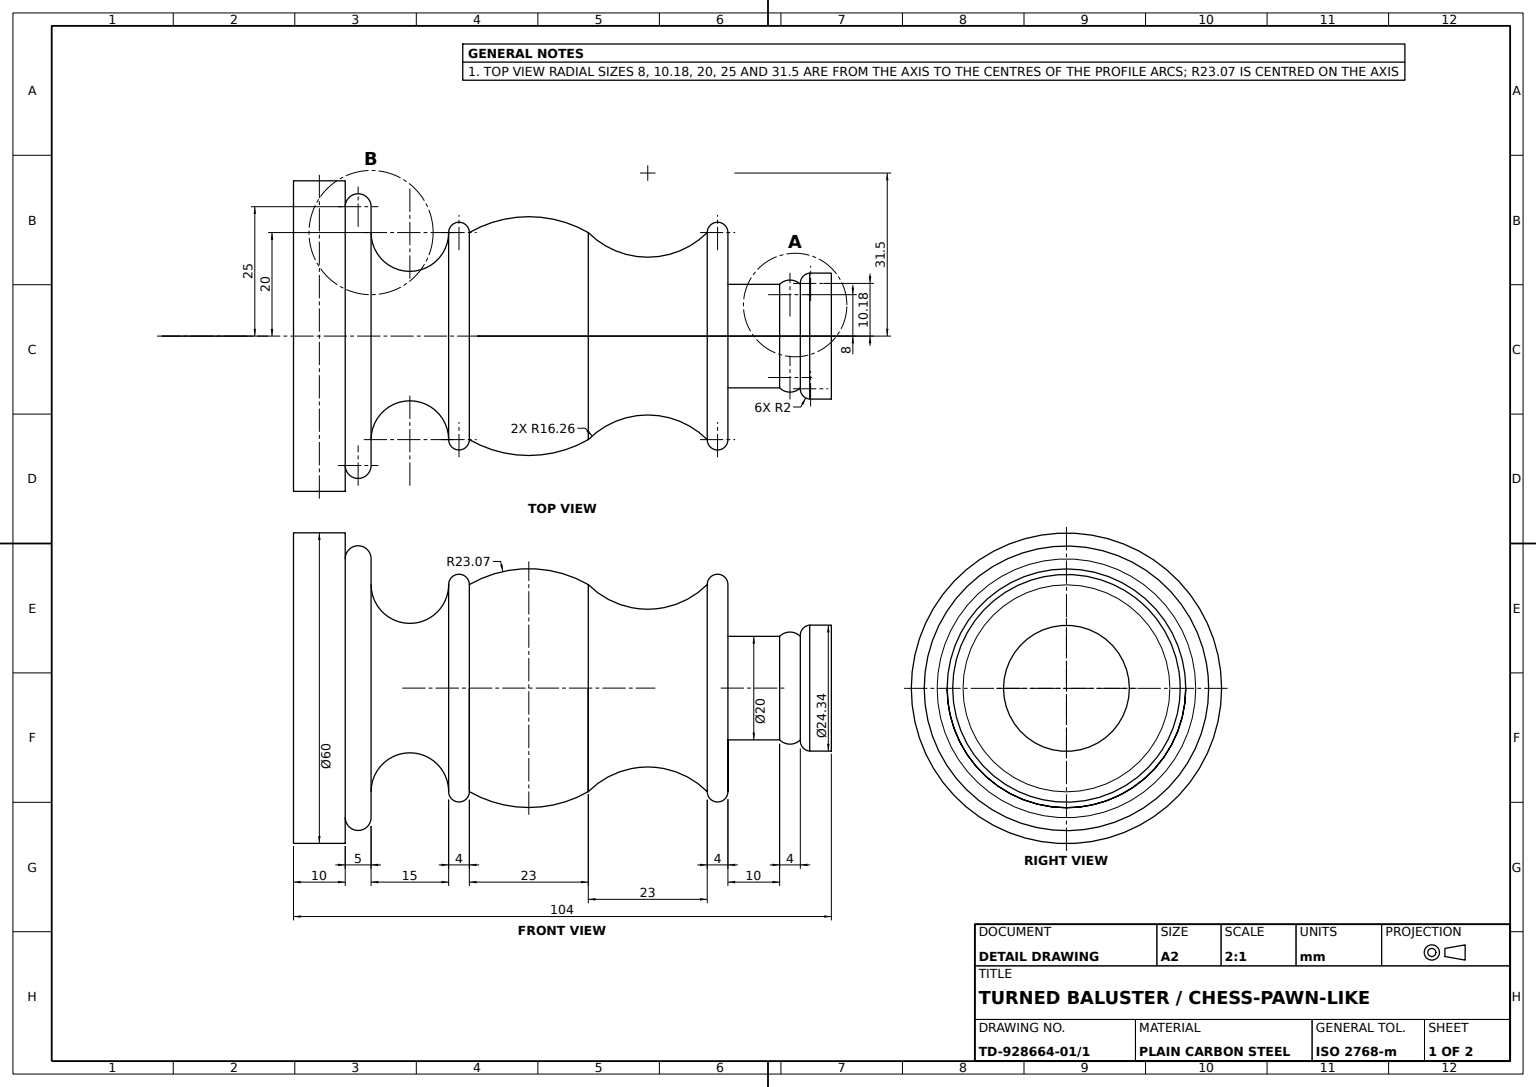
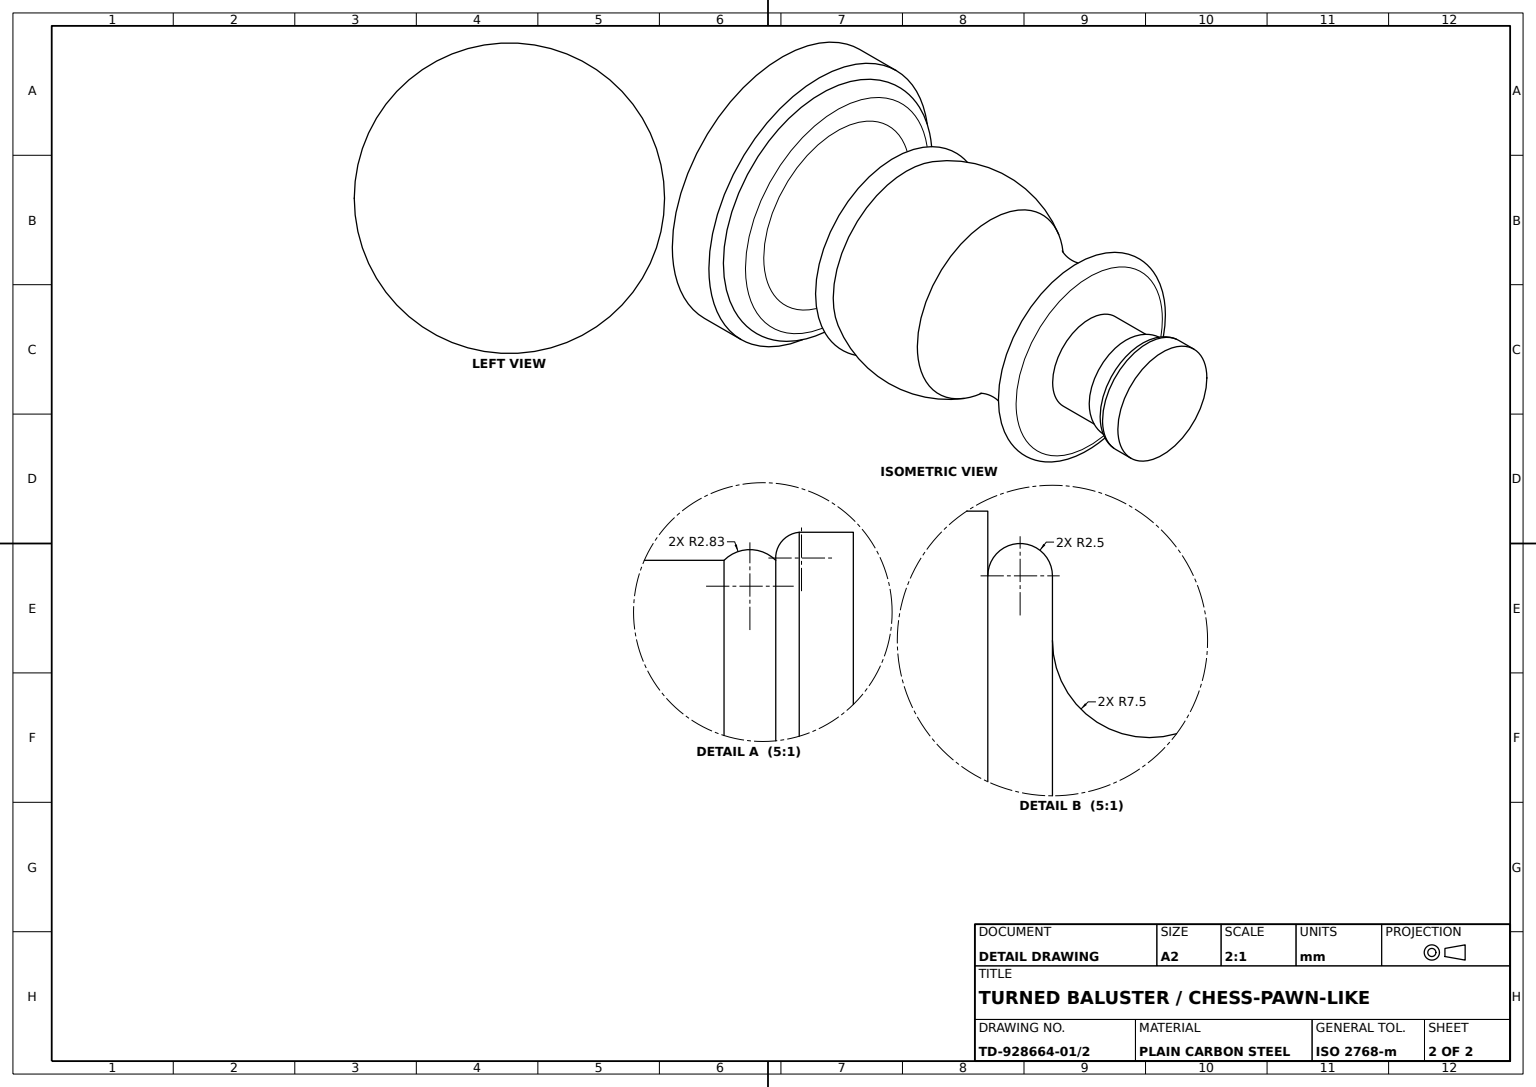
from build123d import *


with BuildPart() as part:
    # Baluster Half Profile → Baluster Body Revolve 360° (revolve)
    with BuildSketch(Plane.XY, mode=Mode.PRIVATE) as baluster_body_revolve_360_sk:
        with BuildLine():
            Line((0, 0), (30, 0))
            Line((30, 0), (30, 10))
            Line((30, 10), (25, 10))
            ThreePointArc((25, 10), (27.5, 12.5), (25, 15))
            Line((25, 15), (20, 15))
            ThreePointArc((20, 15), (12.5, 22.5), (20, 30))
            ThreePointArc((20, 30), (22, 32), (20, 34))
            ThreePointArc((20, 34), (23.07054399, 45.5), (20, 57))
            ThreePointArc((20, 57), (15.236544033, 68.5), (20, 80))
            ThreePointArc((20, 80), (22, 82), (20, 84))
            Line((20, 84), (10, 84))
            Line((10, 84), (10, 94))
            ThreePointArc((10, 94), (10.828427125, 96), (10, 98))
            Line((10, 98), (10.353016606, 98))
            ThreePointArc((10.353016606, 98), (11.590721865, 98.577982417), (12.168704282, 99.815687676))
            Line((12.168704282, 99.815687676), (12.168704282, 104))
            Line((12.168704282, 104), (0, 104))
            Line((0, 104), (0, 0))
        make_face()
    revolve(baluster_body_revolve_360_sk.sketch.rotate(Axis((0, 0, 0), (0, 1, 0)), 90), axis=Axis((0, 0, 0), (0, 1, 0)))


solid = part.part
